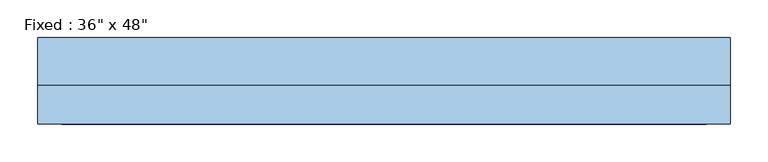
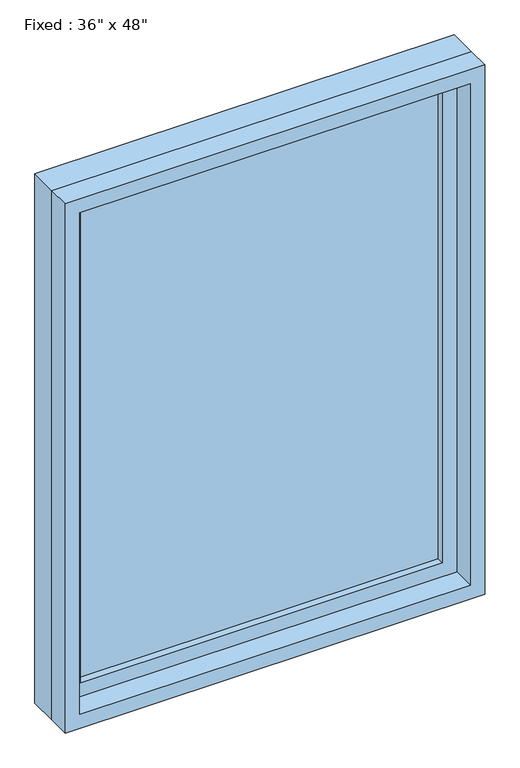
"""IFC4 building model written with IfcOpenShell, lengths in millimetres: window geometry."""

from ifc_helpers import new_model, si_unit, frame, origin, place, context, project, spatial, polyline, outline, extrude, source, transform, mapped, element, save


def window_41a96561(model_context):
    return source(origin(), model_context, "Body", "SweptSolid", [
        extrude(outline(polyline([(355.6, 9.525), (-431.8, 9.525), (-431.8, 22.225), (355.6, 22.225), (355.6, 9.525)])), frame((0.0, 0.0, 977.9), z_axis=(0.0, 0.0, 1.0), x_axis=(1.0, 0.0, 0.0)), (0.0, 0.0, 1.0), 1092.2),
        extrude(outline(polyline([(2114.55, -476.25), (933.45, -476.25), (933.45, 400.05), (2114.55, 400.05), (2114.55, -476.25)]), holes=[polyline([(2070.1, -431.8), (2070.1, 355.6), (977.9, 355.6), (977.9, -431.8), (2070.1, -431.8)])]), frame((0.0, -6.35, 0.0), z_axis=(0.0, 1.0, 0.0), x_axis=(0.0, 0.0, 1.0)), (0.0, 0.0, 1.0), 44.45),
        extrude(outline(polyline([(2133.6, -495.3), (914.4, -495.3), (914.4, 419.1), (2133.6, 419.1), (2133.6, -495.3)]), holes=[polyline([(2101.85, -463.55), (2101.85, 387.35), (946.15, 387.35), (946.15, -463.55), (2101.85, -463.55)])]), frame((0.0, -57.15, 0.0), z_axis=(0.0, 1.0, 0.0), x_axis=(0.0, 0.0, 1.0)), (0.0, 0.0, 1.0), 50.8),
        extrude(outline(polyline([(2133.6, 419.1), (2133.6, -495.3), (914.4, -495.3), (914.4, 419.1), (2133.6, 419.1)]), holes=[polyline([(2114.55, 400.05), (933.45, 400.05), (933.45, -476.25), (2114.55, -476.25), (2114.55, 400.05)])]), frame((0.0, -6.35, 0.0), z_axis=(0.0, 1.0, 0.0), x_axis=(0.0, 0.0, 1.0)), (0.0, 0.0, 1.0), 63.5),
    ])


if __name__ == "__main__":
    model = new_model("IFC4")
    model_context = context("Model", 3, world=origin())
    ifc_project = project(units=[si_unit("LENGTHUNIT", "METRE", prefix="MILLI")], contexts=[model_context])
    site = spatial("IfcSite", under=ifc_project)
    building = spatial("IfcBuilding", under=site)
    placement = place(None, origin())
    window_shape = window_41a96561(model_context)
    element("IfcWindow", 1, ObjectType="Fixed : 36\" x 48\"", at=placement, inside=building, context=model_context, shape_type="MappedRepresentation", body=[
        mapped(window_shape, transform((0.0, 0.0, 0.0), x_axis=(1.0, 0.0, 0.0), y_axis=(0.0, 1.0, 0.0), z_axis=(0.0, 0.0, 1.0))),
    ])
    save(model, "model.ifc")

# Revit data of these elements
# Type "Fixed : 36\" x 48\""
#   Type Mark = "1"
#   Construction Type Id = "GSP4R"
#   Assembly Code = "B2020100"
#   Analytic Construction = "1/8 in Pilkington single glazing"
#   Visual Light Transmittance = 0.9
#   Solar Heat Gain Coefficient = 0.78
#   Heat Transfer Coefficient (U) = 0.6496 BTU/(h·ft²·°F)
#   Height = 4' - 0"
#   Default Sill Height = 3' - 0"
#   Width = 3' - 0"
#   Window Inset = 0' - 0 3/4"
#   Define Thermal Properties by = 1
#   Define Thermal Properties by = 1
#   Glass Pane Material = Glass
#   Sash Material = Sash
#   Wall Closure = (empty or 0)
# Element 1 (IfcWindow, "Fixed : 36\" x 48\"")
#   Materials on its faces: "Sash", "Glass"
# Materials
#   "Glass": class "Glass", colour RGB 0 128 192, transparency 0.75, Description = "Soda Lime Glass", Cost = 0
#   "Sash": class "Wood", colour RGB 224 178 126, transparency 0, Cost = 0
